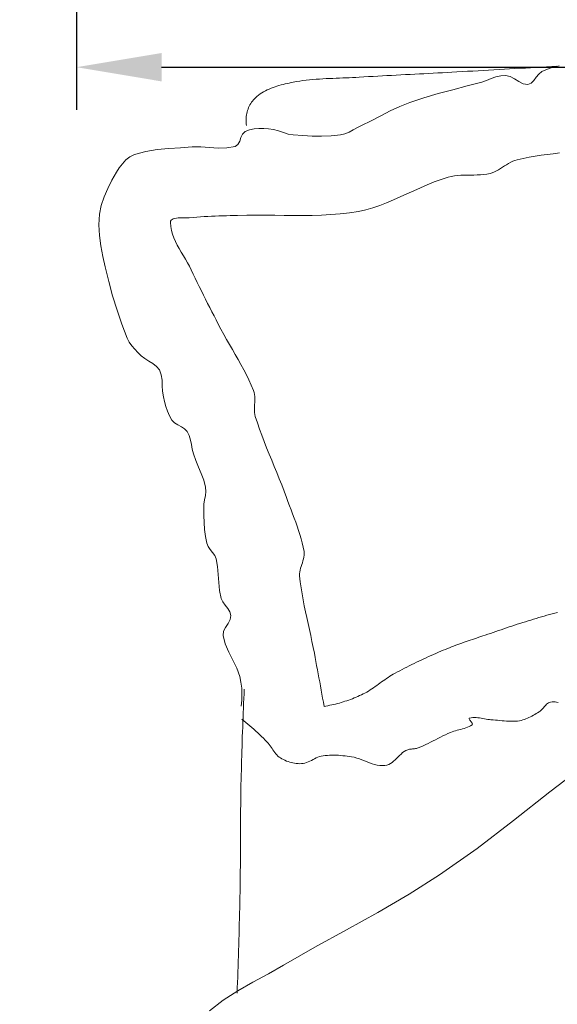
# Model space of a CAD drawing. Units: inches. Extents: x 1484 to 2008, y 1843 to 2590.
# Tile 14 of 21: x 1802 to 1817, y 2172 to 2201. Entities that reach past the tile are written whole.
import ezdxf

# ---------------------------------------------------------------- set-up
doc = ezdxf.new("R2010")
doc.units = ezdxf.units.IN
doc.layers.add('A-ANNO-DIMS', color=2, linetype='Continuous', lineweight=18)
doc.layers.add('A-FURN', color=8, linetype='Continuous', lineweight=18)
doc.styles.get("Standard").update_dxf_attribs({"font": 'arial.ttf'})
doc.dimstyles.new('ISO-25', dxfattribs={"dimtxt": 7, "dimasz": 2.5, "dimexe": 1.25, "dimexo": 0.625, "dimtad": 1, "dimdec": 0, "dimlunit": 3, "dimtxsty": 'Standard', "dimcen": 2.5, "dimadec": 0, "dimazin": 0, "dimtfac": 1, "dimtdec": 0, "dimtmove": 0, "dimatfit": 3, "dimfxl": 1, "dimarcsym": 0})

# ---------------------------------------------------------------- blocks, each defined once
blk = doc.blocks.new('BED-DOUBLE')
for p, q in [((14.395, 80.112), (14.55, 80.121)), ((14.55, 80.121), (14.705, 80.13)), ((14.594, 80.099), (14.766, 80.146)), ((9.167, 79.824), (9.303, 79.832)), ((9.303, 79.832), (9.439, 79.84)), ((9.439, 79.84), (9.574, 79.848)), ((9.574, 79.848), (9.71, 79.855)), ((9.71, 79.855), (9.846, 79.863)), ((9.846, 79.863), (9.982, 79.87)), ((9.982, 79.87), (10.117, 79.877)), ((10.117, 79.877), (10.253, 79.884)), ((10.253, 79.884), (10.389, 79.891)), ((10.389, 79.891), (10.525, 79.898)), ((10.525, 79.898), (10.661, 79.905)), ((10.661, 79.905), (10.796, 79.912)), ((10.796, 79.912), (10.932, 79.92)), ((10.932, 79.92), (11.068, 79.927)), ((11.068, 79.927), (11.204, 79.934)), ((11.204, 79.934), (11.339, 79.941)), ((11.339, 79.941), (11.475, 79.948)), ((11.475, 79.948), (11.611, 79.956)), ((11.611, 79.956), (11.766, 79.964)), ((11.766, 79.964), (11.92, 79.973)), ((11.92, 79.973), (12.075, 79.982)), ((12.075, 79.982), (12.23, 79.99)), ((12.23, 79.99), (12.385, 79.999)), ((12.385, 79.999), (12.539, 80.008)), ((12.539, 80.008), (12.694, 80.016)), ((12.694, 80.016), (12.849, 80.025)), ((12.849, 80.025), (13.003, 80.034)), ((12.91, 79.817), (13.051, 79.853)), ((13.003, 80.034), (13.158, 80.042)), ((13.051, 79.853), (13.195, 79.863)), ((13.158, 80.042), (13.313, 80.051)), ((13.195, 79.863), (13.33, 79.829)), ((13.313, 80.051), (13.467, 80.06)), ((13.33, 79.829), (13.458, 79.758)), ((13.467, 80.06), (13.622, 80.069)), ((13.622, 80.069), (13.777, 80.077)), ((13.777, 80.077), (13.931, 80.086)), ((13.931, 80.086), (14.086, 80.095)), ((14.086, 80.095), (14.241, 80.104)), ((14.097, 79.81), (14.174, 79.902)), ((14.174, 79.902), (14.264, 79.971)), ((14.241, 80.104), (14.395, 80.112)), ((14.264, 79.971), (14.426, 80.042)), ((14.426, 80.042), (14.594, 80.099)), ((6.421, 79.527), (6.479, 79.546)), ((6.479, 79.546), (6.538, 79.563)), ((6.538, 79.563), (6.598, 79.58)), ((6.598, 79.58), (6.657, 79.596)), ((6.657, 79.596), (6.717, 79.61)), ((6.717, 79.61), (6.777, 79.624)), ((6.777, 79.624), (6.836, 79.637)), ((6.836, 79.637), (6.896, 79.649)), ((6.896, 79.649), (6.955, 79.661)), ((6.955, 79.661), (7.05, 79.679)), ((7.05, 79.679), (7.146, 79.695)), ((7.146, 79.695), (7.242, 79.709)), ((7.242, 79.709), (7.339, 79.721)), ((7.339, 79.721), (7.436, 79.731)), ((7.436, 79.731), (7.532, 79.74)), ((7.532, 79.74), (7.629, 79.748)), ((7.629, 79.748), (7.726, 79.755)), ((7.726, 79.755), (7.824, 79.761)), ((7.824, 79.761), (7.921, 79.766)), ((7.921, 79.766), (8.019, 79.77)), ((8.019, 79.77), (8.116, 79.774)), ((8.116, 79.774), (8.214, 79.778)), ((8.214, 79.778), (8.311, 79.781)), ((8.311, 79.781), (8.409, 79.785)), ((8.409, 79.785), (8.506, 79.788)), ((8.506, 79.788), (8.604, 79.792)), ((8.604, 79.792), (8.701, 79.797)), ((8.701, 79.797), (8.798, 79.802)), ((8.798, 79.802), (8.896, 79.807)), ((8.896, 79.807), (9.031, 79.816)), ((9.031, 79.816), (9.167, 79.824)), ((11.642, 79.44), (12.068, 79.55)), ((12.068, 79.55), (12.492, 79.664)), ((12.492, 79.664), (12.631, 79.711)), ((12.631, 79.711), (12.771, 79.766)), ((12.771, 79.766), (12.91, 79.817)), ((13.458, 79.758), (13.583, 79.678)), ((13.583, 79.678), (13.71, 79.616)), ((13.71, 79.616), (13.844, 79.598)), ((13.844, 79.598), (13.943, 79.636)), ((13.943, 79.636), (14.024, 79.714)), ((14.024, 79.714), (14.097, 79.81)), ((5.89, 79.245), (5.937, 79.282)), ((5.937, 79.282), (5.986, 79.317)), ((5.986, 79.317), (6.036, 79.35)), ((6.036, 79.35), (6.087, 79.381)), ((6.087, 79.381), (6.14, 79.409)), ((6.14, 79.409), (6.194, 79.436)), ((6.194, 79.436), (6.25, 79.461)), ((6.25, 79.461), (6.306, 79.485)), ((6.306, 79.485), (6.363, 79.506)), ((6.363, 79.506), (6.421, 79.527)), ((10.796, 79.207), (11.218, 79.329)), ((11.218, 79.329), (11.642, 79.44)), ((5.647, 78.916), (5.665, 78.957)), ((5.665, 78.957), (5.686, 78.997)), ((5.686, 78.997), (5.708, 79.036)), ((5.708, 79.036), (5.732, 79.074)), ((5.732, 79.074), (5.758, 79.109)), ((5.758, 79.109), (5.786, 79.143)), ((5.786, 79.143), (5.815, 79.176)), ((5.815, 79.176), (5.845, 79.206)), ((5.845, 79.206), (5.89, 79.245)), ((10.089, 78.952), (10.38, 79.069)), ((10.38, 79.069), (10.796, 79.207)), ((5.576, 78.654), (5.583, 78.699)), ((5.583, 78.699), (5.591, 78.743)), ((5.591, 78.743), (5.602, 78.787)), ((5.602, 78.787), (5.615, 78.831)), ((5.615, 78.831), (5.63, 78.874)), ((5.63, 78.874), (5.647, 78.916)), ((9.245, 78.531), (9.525, 78.675)), ((9.525, 78.675), (9.805, 78.818)), ((9.805, 78.818), (10.089, 78.952)), ((5.57, 78.565), (5.572, 78.61)), ((5.57, 78.521), (5.57, 78.565)), ((5.573, 78.477), (5.57, 78.521)), ((5.572, 78.61), (5.576, 78.654)), ((5.578, 78.434), (5.573, 78.477)), ((5.585, 78.392), (5.578, 78.434)), ((8.842, 78.329), (8.963, 78.392)), ((8.963, 78.392), (9.245, 78.531)), ((5.421, 78.035), (5.467, 78.138)), ((5.467, 78.138), (5.54, 78.21)), ((5.54, 78.21), (5.668, 78.261)), ((5.668, 78.261), (5.805, 78.29)), ((5.805, 78.29), (5.946, 78.301)), ((5.946, 78.301), (6.089, 78.3)), ((6.089, 78.3), (6.23, 78.292)), ((6.23, 78.292), (6.378, 78.269)), ((6.378, 78.269), (6.523, 78.228)), ((6.523, 78.228), (6.667, 78.18)), ((6.667, 78.18), (6.812, 78.138)), ((6.812, 78.138), (6.959, 78.112)), ((6.959, 78.112), (7.236, 78.091)), ((7.236, 78.091), (7.514, 78.077)), ((8.068, 78.085), (8.344, 78.113)), ((8.344, 78.113), (8.475, 78.145)), ((8.475, 78.145), (8.6, 78.197)), ((8.6, 78.197), (8.721, 78.261)), ((8.721, 78.261), (8.842, 78.329)), ((5.254, 77.774), (5.333, 77.83)), ((5.333, 77.83), (5.383, 77.925)), ((5.383, 77.925), (5.421, 78.035)), ((7.514, 78.077), (7.791, 78.074)), ((7.791, 78.074), (8.068, 78.085)), ((2.16, 77.473), (2.294, 77.537)), ((2.294, 77.537), (2.622, 77.626)), ((2.622, 77.626), (2.959, 77.681)), ((2.959, 77.681), (3.3, 77.714)), ((3.3, 77.714), (3.644, 77.737)), ((3.644, 77.737), (3.985, 77.76)), ((3.985, 77.76), (4.24, 77.763)), ((4.24, 77.763), (4.497, 77.746)), ((4.497, 77.746), (4.753, 77.728)), ((4.753, 77.728), (5.007, 77.731)), ((5.007, 77.731), (5.254, 77.774)), ((14.062, 77.489), (14.24, 77.515)), ((14.24, 77.515), (14.418, 77.54)), ((14.418, 77.54), (14.596, 77.562)), ((14.596, 77.562), (14.774, 77.584)), ((1.843, 77.143), (1.936, 77.268)), ((1.936, 77.268), (2.041, 77.381)), ((2.041, 77.381), (2.16, 77.473)), ((13.166, 77.202), (13.225, 77.239)), ((13.225, 77.239), (13.285, 77.275)), ((13.285, 77.275), (13.345, 77.308)), ((13.345, 77.308), (13.407, 77.338)), ((13.407, 77.338), (13.47, 77.363)), ((13.47, 77.363), (13.536, 77.383)), ((13.536, 77.383), (13.71, 77.423)), ((13.71, 77.423), (13.886, 77.458)), ((13.886, 77.458), (14.062, 77.489)), ((1.63, 76.781), (1.762, 77.014)), ((1.762, 77.014), (1.843, 77.143)), ((11.976, 76.931), (12.072, 76.933)), ((12.072, 76.933), (12.168, 76.933)), ((12.168, 76.933), (12.265, 76.934)), ((12.265, 76.934), (12.361, 76.937)), ((12.361, 76.937), (12.456, 76.942)), ((12.456, 76.942), (12.551, 76.951)), ((12.551, 76.951), (12.645, 76.964)), ((12.645, 76.964), (12.738, 76.984)), ((12.738, 76.984), (12.803, 77.004)), ((12.803, 77.004), (12.867, 77.029)), ((12.867, 77.029), (12.929, 77.059)), ((12.929, 77.059), (12.989, 77.092)), ((12.989, 77.092), (13.049, 77.127)), ((13.049, 77.127), (13.108, 77.164)), ((13.108, 77.164), (13.166, 77.202)), ((1.506, 76.542), (1.63, 76.781)), ((10.694, 76.563), (10.894, 76.65)), ((10.894, 76.65), (11.095, 76.732)), ((11.095, 76.732), (11.299, 76.806)), ((11.299, 76.806), (11.505, 76.872)), ((11.505, 76.872), (11.597, 76.894)), ((11.597, 76.894), (11.69, 76.911)), ((11.69, 76.911), (11.785, 76.922)), ((11.785, 76.922), (11.88, 76.928)), ((11.88, 76.928), (11.976, 76.931)), ((1.398, 76.295), (1.506, 76.542)), ((10.1, 76.29), (10.298, 76.381)), ((10.298, 76.381), (10.496, 76.473)), ((10.496, 76.473), (10.694, 76.563)), ((1.315, 76.042), (1.398, 76.295)), ((9.499, 76.041), (9.701, 76.118)), ((9.701, 76.118), (9.901, 76.202)), ((9.901, 76.202), (10.1, 76.29)), ((1.249, 75.472), (1.265, 75.782)), ((1.265, 75.782), (1.315, 76.042)), ((8.063, 75.771), (8.335, 75.794)), ((8.335, 75.794), (8.606, 75.825)), ((8.606, 75.825), (8.876, 75.868)), ((8.876, 75.868), (9.087, 75.914)), ((9.087, 75.914), (9.295, 75.972)), ((9.295, 75.972), (9.499, 76.041)), ((3.347, 75.536), (3.352, 75.576)), ((3.358, 75.421), (3.347, 75.536)), ((3.352, 75.576), (3.369, 75.608)), ((3.369, 75.608), (3.397, 75.632)), ((3.397, 75.632), (3.433, 75.65)), ((3.433, 75.65), (3.476, 75.662)), ((3.476, 75.662), (3.525, 75.67)), ((3.525, 75.67), (3.579, 75.675)), ((3.579, 75.675), (3.635, 75.677)), ((3.635, 75.677), (3.693, 75.677)), ((3.693, 75.677), (3.75, 75.677)), ((3.75, 75.677), (3.805, 75.677)), ((3.805, 75.677), (3.857, 75.678)), ((3.857, 75.678), (3.904, 75.682)), ((3.904, 75.682), (4.013, 75.692)), ((4.013, 75.692), (4.121, 75.701)), ((4.121, 75.701), (4.23, 75.709)), ((4.23, 75.709), (4.339, 75.716)), ((4.339, 75.716), (4.448, 75.721)), ((4.448, 75.721), (4.557, 75.726)), ((4.557, 75.726), (4.666, 75.729)), ((4.666, 75.729), (4.775, 75.733)), ((4.775, 75.733), (4.884, 75.736)), ((4.884, 75.736), (4.993, 75.739)), ((4.993, 75.739), (5.102, 75.742)), ((5.102, 75.742), (5.211, 75.745)), ((5.211, 75.745), (5.32, 75.749)), ((5.32, 75.749), (5.594, 75.756)), ((5.594, 75.756), (5.868, 75.759)), ((5.868, 75.759), (6.143, 75.757)), ((6.143, 75.757), (6.418, 75.754)), ((6.418, 75.754), (6.693, 75.75)), ((6.693, 75.75), (6.967, 75.747)), ((6.967, 75.747), (7.242, 75.746)), ((7.242, 75.746), (7.516, 75.749)), ((7.516, 75.749), (7.79, 75.757)), ((7.79, 75.757), (8.063, 75.771)), ((1.266, 75.162), (1.249, 75.472)), ((3.379, 75.308), (3.358, 75.421)), ((3.411, 75.198), (3.379, 75.308)), ((3.451, 75.09), (3.411, 75.198)), ((1.309, 74.851), (1.266, 75.162)), ((3.498, 74.983), (3.451, 75.09)), ((3.551, 74.878), (3.498, 74.983)), ((1.368, 74.543), (1.309, 74.851)), ((3.607, 74.773), (3.551, 74.878)), ((3.667, 74.669), (3.607, 74.773)), ((3.728, 74.566), (3.667, 74.669)), ((1.435, 74.237), (1.368, 74.543)), ((3.789, 74.463), (3.728, 74.566)), ((3.849, 74.359), (3.789, 74.463)), ((3.906, 74.255), (3.849, 74.359)), ((1.537, 73.811), (1.435, 74.237)), ((3.958, 74.15), (3.906, 74.255)), ((4.017, 74.026), (3.958, 74.15)), ((1.652, 73.387), (1.537, 73.811)), ((4.076, 73.903), (4.017, 74.026)), ((4.136, 73.779), (4.076, 73.903)), ((4.196, 73.656), (4.136, 73.779)), ((4.257, 73.533), (4.196, 73.656)), ((4.319, 73.41), (4.257, 73.533)), ((1.78, 72.968), (1.652, 73.387)), ((4.38, 73.288), (4.319, 73.41)), ((4.442, 73.165), (4.38, 73.288)), ((1.922, 72.553), (1.78, 72.968)), ((4.504, 73.043), (4.442, 73.165)), ((4.567, 72.921), (4.504, 73.043)), ((4.629, 72.799), (4.567, 72.921)), ((4.692, 72.677), (4.629, 72.799)), ((4.755, 72.555), (4.692, 72.677)), ((2.079, 72.144), (1.922, 72.553)), ((4.834, 72.404), (4.755, 72.555)), ((4.916, 72.255), (4.834, 72.404)), ((2.138, 72.026), (2.079, 72.144)), ((2.213, 71.918), (2.138, 72.026)), ((5, 72.107), (4.916, 72.255)), ((5.084, 71.959), (5, 72.107)), ((2.299, 71.816), (2.213, 71.918)), ((2.392, 71.72), (2.299, 71.816)), ((5.17, 71.811), (5.084, 71.959)), ((5.255, 71.664), (5.17, 71.811)), ((2.487, 71.626), (2.392, 71.72)), ((2.594, 71.541), (2.487, 71.626)), ((2.715, 71.469), (2.594, 71.541)), ((2.835, 71.397), (2.715, 71.469)), ((5.339, 71.515), (5.255, 71.664)), ((5.422, 71.367), (5.339, 71.515)), ((2.942, 71.315), (2.835, 71.397)), ((3.024, 71.211), (2.942, 71.315)), ((3.079, 71.064), (3.024, 71.211)), ((5.502, 71.217), (5.422, 71.367)), ((5.58, 71.066), (5.502, 71.217)), ((3.102, 70.907), (3.079, 71.064)), ((3.11, 70.744), (3.102, 70.907)), ((5.655, 70.914), (5.58, 71.066)), ((5.725, 70.759), (5.655, 70.914)), ((3.118, 70.581), (3.11, 70.744)), ((3.142, 70.423), (3.118, 70.581)), ((5.791, 70.603), (5.725, 70.759)), ((5.809, 70.548), (5.791, 70.603)), ((3.177, 70.28), (3.142, 70.423)), ((5.821, 70.491), (5.809, 70.548)), ((5.827, 70.434), (5.821, 70.491)), ((5.826, 70.257), (5.829, 70.316)), ((5.83, 70.375), (5.827, 70.434)), ((5.829, 70.316), (5.83, 70.375)), ((3.215, 70.137), (3.177, 70.28)), ((3.26, 69.997), (3.215, 70.137)), ((3.317, 69.862), (3.26, 69.997)), ((5.817, 70.077), (5.819, 70.137)), ((5.817, 70.018), (5.817, 70.077)), ((5.82, 69.96), (5.817, 70.018)), ((5.819, 70.137), (5.822, 70.197)), ((5.822, 70.197), (5.826, 70.257)), ((3.39, 69.737), (3.317, 69.862)), ((3.468, 69.657), (3.39, 69.737)), ((5.829, 69.902), (5.82, 69.96)), ((5.842, 69.846), (5.829, 69.902)), ((5.902, 69.659), (5.842, 69.846)), ((3.566, 69.597), (3.468, 69.657)), ((3.67, 69.543), (3.566, 69.597)), ((3.767, 69.482), (3.67, 69.543)), ((3.843, 69.402), (3.767, 69.482)), ((5.966, 69.473), (5.902, 69.659)), ((6.033, 69.289), (5.966, 69.473)), ((3.902, 69.281), (3.843, 69.402)), ((3.939, 69.151), (3.902, 69.281)), ((3.965, 69.015), (3.939, 69.151)), ((6.103, 69.105), (6.033, 69.289)), ((3.99, 68.879), (3.965, 69.015)), ((4.024, 68.747), (3.99, 68.879)), ((6.175, 68.922), (6.103, 69.105)), ((6.248, 68.74), (6.175, 68.922)), ((4.096, 68.551), (4.024, 68.747)), ((4.176, 68.358), (4.096, 68.551)), ((6.323, 68.558), (6.248, 68.74)), ((6.398, 68.376), (6.323, 68.558)), ((4.256, 68.164), (4.176, 68.358)), ((6.472, 68.195), (6.398, 68.376)), ((4.326, 67.968), (4.256, 68.164)), ((4.377, 67.767), (4.326, 67.968)), ((6.546, 68.012), (6.472, 68.195)), ((6.619, 67.83), (6.546, 68.012)), ((4.386, 67.642), (4.377, 67.767)), ((6.689, 67.646), (6.619, 67.83)), ((4.333, 67.265), (4.353, 67.391)), ((4.353, 67.391), (4.375, 67.517)), ((4.375, 67.517), (4.386, 67.642)), ((6.757, 67.462), (6.689, 67.646)), ((6.802, 67.342), (6.757, 67.462)), ((4.326, 67.139), (4.333, 67.265)), ((4.331, 66.934), (4.326, 67.139)), ((6.847, 67.221), (6.802, 67.342)), ((6.893, 67.101), (6.847, 67.221)), ((6.939, 66.981), (6.893, 67.101)), ((4.338, 66.728), (4.331, 66.934)), ((6.985, 66.86), (6.939, 66.981)), ((7.03, 66.739), (6.985, 66.86)), ((4.352, 66.524), (4.338, 66.728)), ((4.377, 66.32), (4.352, 66.524)), ((7.073, 66.618), (7.03, 66.739)), ((7.115, 66.496), (7.073, 66.618)), ((4.417, 66.12), (4.377, 66.32)), ((7.154, 66.374), (7.115, 66.496)), ((7.19, 66.251), (7.154, 66.374)), ((7.222, 66.127), (7.19, 66.251)), ((4.458, 66.023), (4.417, 66.12)), ((4.52, 65.935), (4.458, 66.023)), ((7.25, 66.002), (7.222, 66.127)), ((7.274, 65.876), (7.25, 66.002)), ((4.588, 65.85), (4.52, 65.935)), ((4.65, 65.762), (4.588, 65.85)), ((4.692, 65.665), (4.65, 65.762)), ((4.735, 65.435), (4.692, 65.665)), ((7.242, 65.603), (7.257, 65.658)), ((7.257, 65.658), (7.27, 65.712)), ((7.27, 65.712), (7.277, 65.767)), ((7.279, 65.821), (7.274, 65.876)), ((7.277, 65.767), (7.279, 65.821)), ((4.756, 65.2), (4.735, 65.435)), ((7.156, 65.33), (7.17, 65.385)), ((7.17, 65.385), (7.186, 65.439)), ((7.186, 65.439), (7.205, 65.494)), ((7.205, 65.494), (7.224, 65.548)), ((7.224, 65.548), (7.242, 65.603)), ((4.771, 64.964), (4.756, 65.2)), ((7.141, 65.22), (7.146, 65.275)), ((7.143, 65.165), (7.141, 65.22)), ((7.163, 64.987), (7.143, 65.165)), ((7.146, 65.275), (7.156, 65.33)), ((4.792, 64.729), (4.771, 64.964)), ((7.188, 64.811), (7.163, 64.987)), ((7.216, 64.634), (7.188, 64.811)), ((4.836, 64.499), (4.792, 64.729)), ((4.884, 64.393), (4.836, 64.499)), ((7.248, 64.459), (7.216, 64.634)), ((4.957, 64.296), (4.884, 64.393)), ((5.035, 64.202), (4.957, 64.296)), ((7.282, 64.283), (7.248, 64.459)), ((7.317, 64.108), (7.282, 64.283)), ((5.098, 64.104), (5.035, 64.202)), ((5.128, 63.995), (5.098, 64.104)), ((5.105, 63.874), (5.128, 63.995)), ((7.355, 63.934), (7.317, 64.108)), ((7.393, 63.759), (7.355, 63.934)), ((14.176, 63.935), (14.096, 63.912)), ((14.254, 63.958), (14.176, 63.935)), ((14.332, 63.98), (14.254, 63.958)), ((14.41, 64.002), (14.332, 63.98)), ((14.489, 64.024), (14.41, 64.002)), ((14.567, 64.045), (14.489, 64.024)), ((14.645, 64.067), (14.567, 64.045)), ((14.723, 64.088), (14.645, 64.067)), ((4.909, 63.533), (4.967, 63.647)), ((4.967, 63.647), (5.042, 63.759)), ((5.042, 63.759), (5.105, 63.874)), ((7.432, 63.584), (7.393, 63.759)), ((13.222, 63.633), (13.143, 63.607)), ((13.301, 63.66), (13.222, 63.633)), ((13.381, 63.686), (13.301, 63.66)), ((13.46, 63.712), (13.381, 63.686)), ((13.539, 63.738), (13.46, 63.712)), ((13.618, 63.764), (13.539, 63.738)), ((13.698, 63.789), (13.618, 63.764)), ((13.777, 63.814), (13.698, 63.789)), ((13.857, 63.839), (13.777, 63.814)), ((13.937, 63.864), (13.857, 63.839)), ((14.016, 63.888), (13.937, 63.864)), ((14.096, 63.912), (14.016, 63.888)), ((4.895, 63.413), (4.909, 63.533)), ((4.96, 63.162), (4.895, 63.413)), ((7.47, 63.41), (7.432, 63.584)), ((7.507, 63.235), (7.47, 63.41)), ((12.405, 63.356), (12.344, 63.335)), ((12.467, 63.377), (12.405, 63.356)), ((12.529, 63.398), (12.467, 63.377)), ((12.59, 63.419), (12.529, 63.398)), ((12.669, 63.446), (12.59, 63.419)), ((12.748, 63.472), (12.669, 63.446)), ((12.827, 63.499), (12.748, 63.472)), ((12.906, 63.526), (12.827, 63.499)), ((12.985, 63.553), (12.906, 63.526)), ((13.064, 63.58), (12.985, 63.553)), ((13.143, 63.607), (13.064, 63.58)), ((5.064, 62.923), (4.96, 63.162)), ((7.543, 63.06), (7.507, 63.235)), ((7.577, 62.885), (7.543, 63.06)), ((11.546, 63.051), (11.486, 63.027)), ((11.607, 63.074), (11.546, 63.051)), ((11.668, 63.098), (11.607, 63.074)), ((11.729, 63.12), (11.668, 63.098)), ((11.79, 63.143), (11.729, 63.12)), ((11.851, 63.165), (11.79, 63.143)), ((11.912, 63.187), (11.851, 63.165)), ((11.974, 63.209), (11.912, 63.187)), ((12.035, 63.23), (11.974, 63.209)), ((12.097, 63.251), (12.035, 63.23)), ((12.158, 63.272), (12.097, 63.251)), ((12.22, 63.293), (12.158, 63.272)), ((12.282, 63.314), (12.22, 63.293)), ((12.344, 63.335), (12.282, 63.314)), ((5.185, 62.688), (5.064, 62.923)), ((7.6, 62.765), (7.577, 62.885)), ((7.622, 62.645), (7.6, 62.765)), ((10.934, 62.788), (10.862, 62.755)), ((11.005, 62.82), (10.934, 62.788)), ((11.077, 62.852), (11.005, 62.82)), ((11.149, 62.884), (11.077, 62.852)), ((11.221, 62.915), (11.149, 62.884)), ((11.293, 62.946), (11.221, 62.915)), ((11.365, 62.977), (11.293, 62.946)), ((11.425, 63.002), (11.365, 62.977)), ((11.486, 63.027), (11.425, 63.002)), ((5.3, 62.451), (5.185, 62.688)), ((7.644, 62.525), (7.622, 62.645)), ((7.667, 62.405), (7.644, 62.525)), ((10.296, 62.482), (10.226, 62.447)), ((10.366, 62.518), (10.296, 62.482)), ((10.436, 62.553), (10.366, 62.518)), ((10.507, 62.587), (10.436, 62.553)), ((10.577, 62.622), (10.507, 62.587)), ((10.648, 62.656), (10.577, 62.622)), ((10.719, 62.689), (10.648, 62.656)), ((10.791, 62.722), (10.719, 62.689)), ((10.862, 62.755), (10.791, 62.722)), ((5.386, 62.205), (5.3, 62.451)), ((5.422, 62.034), (5.386, 62.205)), ((7.689, 62.285), (7.667, 62.405)), ((7.711, 62.166), (7.689, 62.285)), ((9.797, 62.21), (9.747, 62.178)), ((9.846, 62.241), (9.797, 62.21)), ((9.897, 62.271), (9.846, 62.241)), ((9.948, 62.3), (9.897, 62.271)), ((10.017, 62.337), (9.948, 62.3)), ((10.087, 62.374), (10.017, 62.337)), ((10.156, 62.41), (10.087, 62.374)), ((10.226, 62.447), (10.156, 62.41)), ((5.444, 61.859), (5.422, 62.034)), ((7.733, 62.046), (7.711, 62.166)), ((7.755, 61.926), (7.733, 62.046)), ((7.776, 61.806), (7.755, 61.926)), ((9.361, 61.907), (9.313, 61.873)), ((9.409, 61.94), (9.361, 61.907)), ((9.457, 61.975), (9.409, 61.94)), ((9.505, 62.009), (9.457, 61.975)), ((9.553, 62.043), (9.505, 62.009)), ((9.601, 62.077), (9.553, 62.043)), ((9.65, 62.111), (9.601, 62.077)), ((9.698, 62.145), (9.65, 62.111)), ((9.747, 62.178), (9.698, 62.145)), ((5.451, 61.683), (5.444, 61.859)), ((5.445, 61.507), (5.451, 61.683)), ((5.505, 61.557), (5.512, 61.697)), ((5.512, 61.697), (5.518, 61.837)), ((7.798, 61.686), (7.776, 61.806)), ((7.82, 61.566), (7.798, 61.686)), ((8.854, 61.619), (8.801, 61.596)), ((8.906, 61.642), (8.854, 61.619)), ((8.958, 61.666), (8.906, 61.642)), ((9.011, 61.691), (8.958, 61.666)), ((9.063, 61.719), (9.011, 61.691)), ((9.114, 61.747), (9.063, 61.719)), ((9.165, 61.777), (9.114, 61.747)), ((9.214, 61.808), (9.165, 61.777)), ((9.264, 61.84), (9.214, 61.808)), ((9.313, 61.873), (9.264, 61.84)), ((5.424, 61.333), (5.445, 61.507)), ((5.493, 61.277), (5.499, 61.417)), ((5.499, 61.417), (5.505, 61.557)), ((7.841, 61.446), (7.82, 61.566)), ((7.863, 61.326), (7.841, 61.446)), ((7.919, 61.336), (7.863, 61.326)), ((7.976, 61.346), (7.919, 61.336)), ((8.032, 61.358), (7.976, 61.346)), ((8.088, 61.37), (8.032, 61.358)), ((8.144, 61.383), (8.088, 61.37)), ((8.2, 61.396), (8.144, 61.383)), ((8.256, 61.411), (8.2, 61.396)), ((8.312, 61.426), (8.256, 61.411)), ((8.367, 61.442), (8.312, 61.426)), ((8.422, 61.459), (8.367, 61.442)), ((8.477, 61.476), (8.422, 61.459)), ((8.532, 61.494), (8.477, 61.476)), ((8.586, 61.513), (8.532, 61.494)), ((8.64, 61.533), (8.586, 61.513)), ((8.694, 61.553), (8.64, 61.533)), ((8.748, 61.574), (8.694, 61.553)), ((8.801, 61.596), (8.748, 61.574)), ((14.353, 61.34), (14.329, 61.313)), ((14.377, 61.366), (14.353, 61.34)), ((14.401, 61.39), (14.377, 61.366)), ((14.428, 61.411), (14.401, 61.39)), ((14.455, 61.43), (14.428, 61.411)), ((14.485, 61.445), (14.455, 61.43)), ((14.517, 61.455), (14.485, 61.445)), ((14.561, 61.462), (14.517, 61.455)), ((14.605, 61.463), (14.561, 61.462)), ((14.649, 61.46), (14.605, 61.463)), ((14.694, 61.452), (14.649, 61.46)), ((14.738, 61.442), (14.694, 61.452)), ((5.482, 60.997), (5.487, 61.137)), ((5.487, 61.137), (5.493, 61.277)), ((13.968, 61.043), (13.925, 61.019)), ((14.01, 61.067), (13.968, 61.043)), ((14.053, 61.091), (14.01, 61.067)), ((14.095, 61.116), (14.053, 61.091)), ((14.136, 61.142), (14.095, 61.116)), ((14.178, 61.167), (14.136, 61.142)), ((14.206, 61.186), (14.178, 61.167)), ((14.233, 61.208), (14.206, 61.186)), ((14.258, 61.233), (14.233, 61.208)), ((14.282, 61.259), (14.258, 61.233)), ((14.306, 61.286), (14.282, 61.259)), ((14.329, 61.313), (14.306, 61.286)), ((5.509, 60.905), (5.449, 60.954)), ((5.471, 60.716), (5.476, 60.856)), ((5.476, 60.856), (5.482, 60.997)), ((5.568, 60.856), (5.509, 60.905)), ((5.627, 60.806), (5.568, 60.856)), ((5.685, 60.755), (5.627, 60.806)), ((5.743, 60.704), (5.685, 60.755)), ((12.167, 60.76), (12.122, 60.735)), ((12.128, 60.979), (12.125, 60.969)), ((12.125, 60.969), (12.128, 60.957)), ((12.139, 60.985), (12.128, 60.979)), ((12.128, 60.957), (12.136, 60.941)), ((12.136, 60.941), (12.148, 60.924)), ((12.186, 60.995), (12.139, 60.985)), ((12.148, 60.924), (12.162, 60.906)), ((12.162, 60.906), (12.177, 60.887)), ((12.21, 60.789), (12.167, 60.76)), ((12.177, 60.887), (12.192, 60.867)), ((12.233, 61), (12.186, 60.995)), ((12.192, 60.867), (12.205, 60.848)), ((12.205, 60.848), (12.215, 60.831)), ((12.218, 60.8), (12.21, 60.789)), ((12.215, 60.831), (12.219, 60.814)), ((12.219, 60.814), (12.218, 60.8)), ((12.281, 61.001), (12.233, 61)), ((12.329, 60.999), (12.281, 61.001)), ((12.377, 60.995), (12.329, 60.999)), ((12.426, 60.988), (12.377, 60.995)), ((12.474, 60.98), (12.426, 60.988)), ((12.523, 60.971), (12.474, 60.98)), ((12.572, 60.961), (12.523, 60.971)), ((12.621, 60.953), (12.572, 60.961)), ((12.669, 60.945), (12.621, 60.953)), ((12.718, 60.939), (12.669, 60.945)), ((12.766, 60.935), (12.718, 60.939)), ((12.831, 60.93), (12.766, 60.935)), ((12.896, 60.925), (12.831, 60.93)), ((12.961, 60.919), (12.896, 60.925)), ((13.026, 60.912), (12.961, 60.919)), ((13.091, 60.906), (13.026, 60.912)), ((13.156, 60.9), (13.091, 60.906)), ((13.221, 60.895), (13.156, 60.9)), ((13.285, 60.891), (13.221, 60.895)), ((13.35, 60.889), (13.285, 60.891)), ((13.415, 60.889), (13.35, 60.889)), ((13.479, 60.892), (13.415, 60.889)), ((13.543, 60.897), (13.479, 60.892)), ((13.607, 60.906), (13.543, 60.897)), ((13.655, 60.915), (13.607, 60.906)), ((13.701, 60.927), (13.655, 60.915)), ((13.747, 60.942), (13.701, 60.927)), ((13.792, 60.958), (13.747, 60.942)), ((13.837, 60.977), (13.792, 60.958)), ((13.881, 60.998), (13.837, 60.977)), ((13.925, 61.019), (13.881, 60.998)), ((5.461, 60.436), (5.466, 60.576)), ((5.466, 60.576), (5.471, 60.716)), ((5.8, 60.653), (5.743, 60.704)), ((5.857, 60.601), (5.8, 60.653)), ((5.914, 60.548), (5.857, 60.601)), ((5.97, 60.496), (5.914, 60.548)), ((6.026, 60.442), (5.97, 60.496)), ((11.353, 60.458), (11.281, 60.422)), ((11.426, 60.493), (11.353, 60.458)), ((11.499, 60.527), (11.426, 60.493)), ((11.573, 60.559), (11.499, 60.527)), ((11.621, 60.579), (11.573, 60.559)), ((11.671, 60.595), (11.621, 60.579)), ((11.721, 60.61), (11.671, 60.595)), ((11.773, 60.624), (11.721, 60.61)), ((11.824, 60.637), (11.773, 60.624)), ((11.876, 60.65), (11.824, 60.637)), ((11.927, 60.664), (11.876, 60.65)), ((11.977, 60.679), (11.927, 60.664)), ((12.027, 60.695), (11.977, 60.679)), ((12.075, 60.714), (12.027, 60.695)), ((12.122, 60.735), (12.075, 60.714)), ((5.452, 60.156), (5.456, 60.296)), ((5.456, 60.296), (5.461, 60.436)), ((6.081, 60.389), (6.026, 60.442)), ((6.136, 60.335), (6.081, 60.389)), ((6.191, 60.28), (6.136, 60.335)), ((6.223, 60.246), (6.191, 60.28)), ((6.253, 60.209), (6.223, 60.246)), ((6.281, 60.171), (6.253, 60.209)), ((6.308, 60.132), (6.281, 60.171)), ((10.776, 60.172), (10.702, 60.139)), ((10.849, 60.206), (10.776, 60.172)), ((10.921, 60.241), (10.849, 60.206)), ((10.993, 60.276), (10.921, 60.241)), ((11.065, 60.313), (10.993, 60.276)), ((11.137, 60.349), (11.065, 60.313)), ((11.209, 60.386), (11.137, 60.349)), ((11.281, 60.422), (11.209, 60.386)), ((5.439, 59.735), (5.443, 59.875)), ((5.443, 59.875), (5.447, 60.015)), ((5.447, 60.015), (5.452, 60.156)), ((6.335, 60.092), (6.308, 60.132)), ((6.362, 60.052), (6.335, 60.092)), ((6.389, 60.013), (6.362, 60.052)), ((6.416, 59.974), (6.389, 60.013)), ((6.445, 59.937), (6.416, 59.974)), ((6.476, 59.902), (6.445, 59.937)), ((6.508, 59.869), (6.476, 59.902)), ((6.543, 59.839), (6.508, 59.869)), ((7.832, 59.875), (7.781, 59.865)), ((7.896, 59.883), (7.832, 59.875)), ((7.961, 59.888), (7.896, 59.883)), ((8.026, 59.892), (7.961, 59.888)), ((8.09, 59.894), (8.026, 59.892)), ((8.155, 59.894), (8.09, 59.894)), ((8.22, 59.892), (8.155, 59.894)), ((8.285, 59.889), (8.22, 59.892)), ((8.35, 59.885), (8.285, 59.889)), ((8.415, 59.879), (8.35, 59.885)), ((8.48, 59.873), (8.415, 59.879)), ((8.545, 59.865), (8.48, 59.873)), ((10.079, 59.887), (10.035, 59.843)), ((10.123, 59.928), (10.079, 59.887)), ((10.169, 59.968), (10.123, 59.928)), ((10.217, 60.003), (10.169, 59.968)), ((10.267, 60.033), (10.217, 60.003)), ((10.293, 60.045), (10.267, 60.033)), ((10.319, 60.054), (10.293, 60.045)), ((10.346, 60.061), (10.319, 60.054)), ((10.374, 60.067), (10.346, 60.061)), ((10.402, 60.071), (10.374, 60.067)), ((10.431, 60.074), (10.402, 60.071)), ((10.46, 60.076), (10.431, 60.074)), ((10.489, 60.079), (10.46, 60.076)), ((10.517, 60.082), (10.489, 60.079)), ((10.546, 60.086), (10.517, 60.082)), ((10.574, 60.092), (10.546, 60.086)), ((10.601, 60.099), (10.574, 60.092)), ((10.628, 60.108), (10.601, 60.099)), ((10.702, 60.139), (10.628, 60.108)), ((5.432, 59.454), (5.435, 59.595)), ((5.435, 59.595), (5.439, 59.735)), ((6.581, 59.812), (6.543, 59.839)), ((6.623, 59.786), (6.581, 59.812)), ((6.667, 59.763), (6.623, 59.786)), ((6.712, 59.742), (6.667, 59.763)), ((6.757, 59.722), (6.712, 59.742)), ((6.804, 59.704), (6.757, 59.722)), ((6.852, 59.689), (6.804, 59.704)), ((6.9, 59.676), (6.852, 59.689)), ((6.949, 59.665), (6.9, 59.676)), ((6.998, 59.656), (6.949, 59.665)), ((7.047, 59.65), (6.998, 59.656)), ((7.097, 59.646), (7.047, 59.65)), ((7.146, 59.644), (7.097, 59.646)), ((7.195, 59.645), (7.146, 59.644)), ((7.246, 59.651), (7.195, 59.645)), ((7.297, 59.662), (7.246, 59.651)), ((7.346, 59.677), (7.297, 59.662)), ((7.395, 59.696), (7.346, 59.677)), ((7.443, 59.718), (7.395, 59.696)), ((7.49, 59.741), (7.443, 59.718)), ((7.538, 59.765), (7.49, 59.741)), ((7.586, 59.789), (7.538, 59.765)), ((7.634, 59.812), (7.586, 59.789)), ((7.682, 59.833), (7.634, 59.812)), ((7.731, 59.851), (7.682, 59.833)), ((7.781, 59.865), (7.731, 59.851)), ((8.609, 59.856), (8.545, 59.865)), ((8.673, 59.846), (8.609, 59.856)), ((8.75, 59.831), (8.673, 59.846)), ((8.825, 59.81), (8.75, 59.831)), ((8.901, 59.785), (8.825, 59.81)), ((8.976, 59.757), (8.901, 59.785)), ((9.05, 59.728), (8.976, 59.757)), ((9.125, 59.698), (9.05, 59.728)), ((9.199, 59.67), (9.125, 59.698)), ((9.273, 59.643), (9.199, 59.67)), ((9.348, 59.62), (9.273, 59.643)), ((9.423, 59.602), (9.348, 59.62)), ((9.499, 59.59), (9.423, 59.602)), ((9.575, 59.586), (9.499, 59.59)), ((9.652, 59.59), (9.575, 59.586)), ((9.708, 59.601), (9.652, 59.59)), ((9.76, 59.621), (9.708, 59.601)), ((9.81, 59.647), (9.76, 59.621)), ((9.858, 59.68), (9.81, 59.647)), ((9.903, 59.717), (9.858, 59.68)), ((9.948, 59.757), (9.903, 59.717)), ((9.992, 59.8), (9.948, 59.757)), ((10.035, 59.843), (9.992, 59.8)), ((15.564, 59.638), (14.493, 58.812)), ((5.425, 59.174), (5.428, 59.314)), ((5.428, 59.314), (5.432, 59.454)), ((5.419, 58.884), (5.422, 59.034)), ((5.422, 59.034), (5.425, 59.174)), ((5.415, 58.584), (5.417, 58.734)), ((5.417, 58.734), (5.419, 58.884)), ((14.493, 58.812), (13.43, 57.976)), ((5.412, 58.284), (5.413, 58.434)), ((5.413, 58.434), (5.415, 58.584)), ((5.41, 57.984), (5.411, 58.134)), ((5.411, 58.134), (5.412, 58.284)), ((5.409, 57.834), (5.41, 57.984)), ((13.43, 57.976), (12.356, 57.156)), ((5.408, 57.534), (5.409, 57.684)), ((5.409, 57.684), (5.409, 57.834)), ((5.407, 57.234), (5.408, 57.384)), ((5.408, 57.384), (5.408, 57.534)), ((5.406, 56.934), (5.407, 57.084)), ((5.407, 57.084), (5.407, 57.234)), ((12.356, 57.156), (11.254, 56.374)), ((5.404, 56.634), (5.405, 56.784)), ((5.405, 56.784), (5.406, 56.934)), ((5.401, 56.334), (5.402, 56.484)), ((5.402, 56.484), (5.404, 56.634)), ((5.396, 56.034), (5.399, 56.184)), ((5.399, 56.184), (5.401, 56.334)), ((11.254, 56.374), (10.361, 55.807)), ((5.39, 55.721), (5.393, 55.877)), ((5.393, 55.877), (5.396, 56.034)), ((5.383, 55.407), (5.387, 55.564)), ((5.387, 55.564), (5.39, 55.721)), ((10.361, 55.807), (9.446, 55.275)), ((5.376, 55.094), (5.38, 55.251)), ((5.38, 55.251), (5.383, 55.407)), ((9.446, 55.275), (8.519, 54.762)), ((5.372, 54.937), (5.376, 55.094)), ((5.364, 54.624), (5.368, 54.781)), ((5.368, 54.781), (5.372, 54.937)), ((8.519, 54.762), (7.591, 54.25)), ((5.355, 54.311), (5.359, 54.467)), ((5.359, 54.467), (5.364, 54.624)), ((5.345, 53.997), (5.35, 54.154)), ((5.35, 54.154), (5.355, 54.311)), ((7.591, 54.25), (6.672, 53.725)), ((5.335, 53.684), (5.34, 53.841)), ((5.34, 53.841), (5.345, 53.997)), ((5.325, 53.371), (5.33, 53.527)), ((5.33, 53.527), (5.335, 53.684)), ((6.672, 53.725), (6.226, 53.473)), ((5.319, 53.214), (5.325, 53.371)), ((5.774, 53.228), (5.328, 52.975)), ((6.226, 53.473), (5.774, 53.228)), ((5.328, 52.975), (4.899, 52.699)), ((5.308, 52.901), (5.313, 53.057)), ((5.313, 53.057), (5.319, 53.214)), ((4.899, 52.699), (4.496, 52.387))]:
    blk.add_line(p, q)
blk = doc.blocks.new('*D12')
at = {"layer": 'A-ANNO-DIMS', "color": 0, "lineweight": -2, "transparency": 16777216}
for p, q in [((1798.407, 2117.29), (1798.407, 2180.139)), ((1793.295, 2117.29), (1799.657, 2117.29)), ((1798.407, 2086.463), (1798.407, 2114.79)), ((1793.295, 2083.963), (1799.657, 2083.963))]:
    blk.add_line(p, q, dxfattribs=at)
at = {"layer": 'A-ANNO-DIMS', "color": 0, "transparency": 16777216}
for points in [[(1797.99, 2114.79), (1798.824, 2114.79), (1798.407, 2117.29)], [(1797.99, 2086.463), (1798.824, 2086.463), (1798.407, 2083.963)]]:
    blk.add_solid(points, dxfattribs=at)
at = {"layer": 'Defpoints', "color": 0, "transparency": 16777216}
for p in [(1792.67, 2117.29), (1798.407, 2117.29), (1792.67, 2083.963)]:
    blk.add_point(p, dxfattribs=at)
at = {"layer": 'A-ANNO-DIMS', "color": 0, "transparency": 16777216, "insert": (1794.163, 2149.965), "char_height": 7, "attachment_point": 5, "rotation": 90}
blk.add_mtext('2\'-9 1/2" TYP.', dxfattribs=at)
blk = doc.blocks.new('*D13')
at = {"layer": 'A-ANNO-DIMS', "color": 0, "lineweight": -2, "transparency": 16777216}
for p, q in [((1803.22, 2207.678), (1803.22, 2198.053)), ((1863.22, 2207.678), (1863.22, 2198.053)), ((1805.72, 2199.303), (1860.72, 2199.303)), ((1863.22, 2199.303), (2008.197, 2199.303))]:
    blk.add_line(p, q, dxfattribs=at)
at = {"layer": 'A-ANNO-DIMS', "color": 0, "transparency": 16777216}
for points in [[(1805.72, 2199.72), (1805.72, 2198.886), (1803.22, 2199.303)], [(1860.72, 2199.72), (1860.72, 2198.886), (1863.22, 2199.303)]]:
    blk.add_solid(points, dxfattribs=at)
at = {"layer": 'Defpoints', "color": 0, "transparency": 16777216}
for p in [(1803.22, 2208.303), (1863.22, 2208.303), (1863.22, 2199.303)]:
    blk.add_point(p, dxfattribs=at)
at = {"layer": 'A-ANNO-DIMS', "color": 0, "transparency": 16777216, "insert": (1936.959, 2203.55), "char_height": 7, "attachment_point": 5}
blk.add_mtext('BEDROOM WINDOW 5\'-0" TYP.', dxfattribs=at)

msp = doc.modelspace()

# ---------------------------------------------------------------- block references
at = {"layer": 'A-FURN'}
msp.add_blockref('BED-DOUBLE', (1802.632, 2119.201), dxfattribs=at)

# ---------------------------------------------------------------- dimensions: what is measured, and where the dimension line sits
at = {"layer": 'A-ANNO-DIMS'}
dim = msp.add_linear_dim(base=(1863.22, 2199.303), p1=(1803.22, 2208.303), p2=(1863.22, 2208.303), text='BEDROOM WINDOW <> TYP.', dimstyle='ISO-25', override={"dimdec": 1, "dimlfac": 1, "dimrnd": 0, "dimzin": 1, "dimdsep": 46, "dimlunit": 4, "dimfrac": 2}, dxfattribs=at)
dim.commit()
dim.dimension.update_dxf_attribs({"geometry": '*D13', "text_midpoint": (1936.959, 2203.55)})
dim = msp.add_linear_dim(base=(1798.407, 2117.29), p1=(1792.67, 2083.963), p2=(1792.67, 2117.29), angle=90, text='<> TYP.', dimstyle='ISO-25', override={"dimdec": 1, "dimlfac": 1, "dimrnd": 0, "dimzin": 1, "dimdsep": 46, "dimlunit": 4, "dimfrac": 2}, dxfattribs=at)
dim.commit()
dim.dimension.update_dxf_attribs({"geometry": '*D12', "text_midpoint": (1794.163, 2149.965)})

doc.saveas('drawing.dxf')
